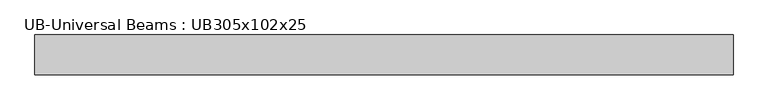
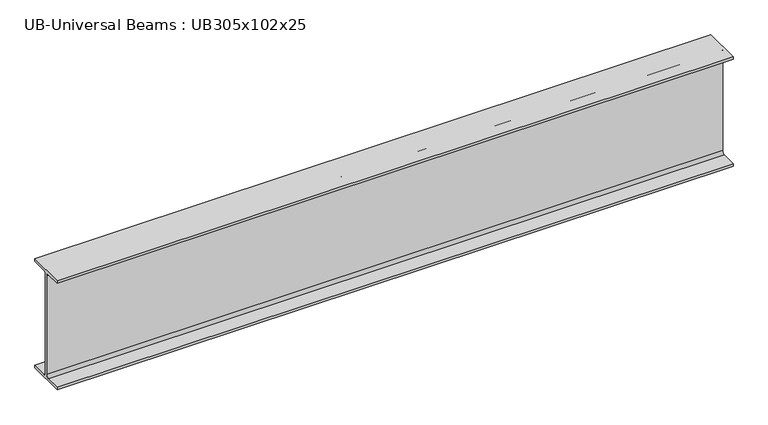
"""IFC4 building model written with IfcOpenShell, lengths in millimetres: beam geometry, UB-Universal Beams : UB305x102x25."""

from ifc_helpers import new_model, si_unit, point, frame, frame_2d, origin, place, context, project, spatial, polyline, circle_curve, trimmed, segment, composite_curve, outline, extrude, source, transform, mapped, element, save


def ub_universal_beams_ub305x102x25_b0bcaaf9(model_context):
    return source(origin(), model_context, "Body", "SweptSolid", [
        extrude(outline(composite_curve([segment(polyline([(50.8, -145.55), (50.8, -152.55), (-50.8, -152.55), (-50.8, -145.55), (-10.5, -145.55)]), True, "CONTINUOUS"), segment(trimmed(circle_curve(frame_2d((-10.5, -137.95)), 7.6), [point((-10.5, -145.55))], [point((-2.9, -137.95))], True, "CARTESIAN"), True, "CONTINUOUS"), segment(polyline([(-2.9, -137.95), (-2.9, 137.95)]), True, "CONTINUOUS"), segment(trimmed(circle_curve(frame_2d((-10.5, 137.95)), 7.6), [point((-2.9, 137.95))], [point((-10.5, 145.55))], True, "CARTESIAN"), True, "CONTINUOUS"), segment(polyline([(-10.5, 145.55), (-50.8, 145.55), (-50.8, 152.55), (50.8, 152.55), (50.8, 145.55), (10.5, 145.55)]), True, "CONTINUOUS"), segment(trimmed(circle_curve(frame_2d((10.5, 137.95)), 7.6), [point((10.5, 145.55))], [point((2.9, 137.95))], True, "CARTESIAN"), True, "CONTINUOUS"), segment(polyline([(2.9, 137.95), (2.9, -137.95)]), True, "CONTINUOUS"), segment(trimmed(circle_curve(frame_2d((10.5, -137.95)), 7.6), [point((2.9, -137.95))], [point((10.5, -145.55))], True, "CARTESIAN"), True, "CONTINUOUS"), segment(polyline([(10.5, -145.55), (50.8, -145.55)]), True, "CONTINUOUS")], self_intersect=False)), frame((-1029.55, 0.0, 0.0), z_axis=(1.0, 0.0, 0.0), x_axis=(0.0, 1.0, 0.0)), (0.0, 0.0, 1.0), 1787.1),
    ])


if __name__ == "__main__":
    model = new_model("IFC4")
    model_context = context("Model", 3, world=origin())
    ifc_project = project(units=[si_unit("LENGTHUNIT", "METRE", prefix="MILLI")], contexts=[model_context])
    site = spatial("IfcSite", under=ifc_project)
    building = spatial("IfcBuilding", under=site)
    placement = place(None, origin())
    ub_universal_beams_ub305x102x25_shape = ub_universal_beams_ub305x102x25_b0bcaaf9(model_context)
    element("IfcBeam", 1, ObjectType="UB-Universal Beams : UB305x102x25", at=placement, inside=building, context=model_context, shape_type="MappedRepresentation", body=[
        mapped(ub_universal_beams_ub305x102x25_shape, transform((0.0, 0.0, 0.0), x_axis=(1.0, 0.0, 0.0), y_axis=(0.0, 1.0, 0.0), z_axis=(0.0, 0.0, 1.0))),
    ])
    save(model, "model.ifc")

# Revit data of these elements
# Type "UB-Universal Beams : UB305x102x25"
#   Section Name Key = "UB305X102X25"
#   Width = 10.16 cm
#   Web Thickness = 0.58 cm
#   Web Fillet = 0.76 cm
#   Warping Constant = 27300.0 cm⁶
#   Torsional Moment of Inertia = 4.77 cm⁴
#   Section Area = 31.6 cm²
#   Plastic Modulus weak axis = 39.0 cm³
#   Plastic Modulus strong axis = 342.0 cm³
#   Nominal Weight = 24.7999 kgf/m
#   Moment of Inertia weak axis = 123.00 cm⁴
#   Moment of Inertia strong axis = 4455.00 cm⁴
#   Height = 30.51 cm
#   Flange Thickness = 0.7 cm
#   Elastic Modulus weak axis = 24.2 cm³
#   Elastic Modulus strong axis = 292.0 cm³
#   Centroid Vertical = 15.255 cm
#   Centroid Horizontal = 5.08 cm
#   Bolt Spacing = 5.4 cm
#   Length [instance default] = 1.5 m
#   Structural Material [instance default] = Metal - Steel 43-275
#   Type Comments = ""
#   Assembly Code = ""
# Element 1 (IfcBeam, "UB-Universal Beams : UB305x102x25")
#   Materials on its faces: "Metal - Steel 43-275"
# Materials
#   "Metal - Steel 43-275": class "Metal", colour RGB 247 247 247, transparency 0, Cost = 0
